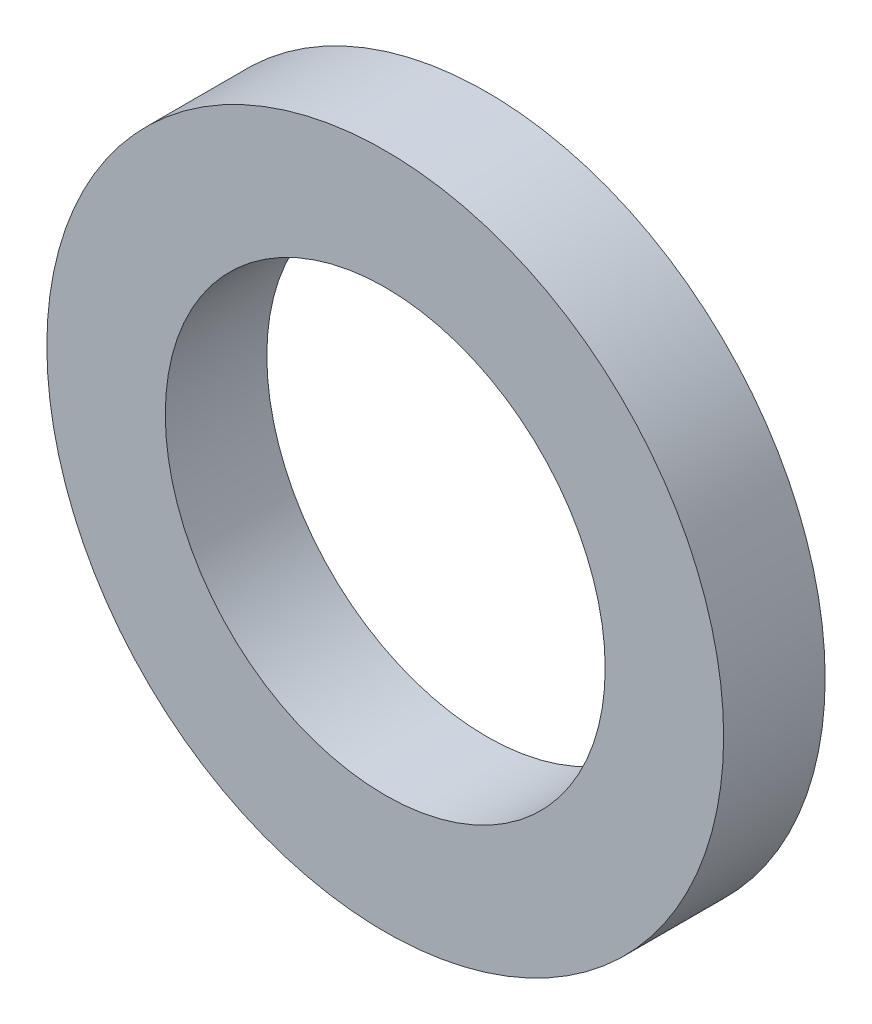
ISO-10303-21;
HEADER;
FILE_DESCRIPTION(('STEP AP214'),'2;1');
FILE_NAME('part.step','',(''),(''),'','','');
FILE_SCHEMA(('AUTOMOTIVE_DESIGN { 1 0 10303 214 1 1 1 1 }'));
ENDSEC;
DATA;
#1=APPLICATION_CONTEXT('core data for automotive mechanical design processes');
#2=APPLICATION_PROTOCOL_DEFINITION('international standard','automotive_design',2000,#1);
#3=PRODUCT_CONTEXT('',#1,'mechanical');
#4=PRODUCT('Part','Part','',(#3));
#5=PRODUCT_RELATED_PRODUCT_CATEGORY('part','',(#4));
#6=PRODUCT_DEFINITION_FORMATION('','',#4);
#7=PRODUCT_DEFINITION_CONTEXT('part definition',#1,'design');
#8=PRODUCT_DEFINITION('design','',#6,#7);
#9=PRODUCT_DEFINITION_SHAPE('','',#8);
#10=(LENGTH_UNIT() NAMED_UNIT(*) SI_UNIT(.MILLI.,.METRE.));
#11=(NAMED_UNIT(*) PLANE_ANGLE_UNIT() SI_UNIT($,.RADIAN.));
#12=(NAMED_UNIT(*) SI_UNIT($,.STERADIAN.) SOLID_ANGLE_UNIT());
#13=UNCERTAINTY_MEASURE_WITH_UNIT(LENGTH_MEASURE(1.E-05),#10,'distance_accuracy_value','');
#14=(GEOMETRIC_REPRESENTATION_CONTEXT(3) GLOBAL_UNCERTAINTY_ASSIGNED_CONTEXT((#13)) GLOBAL_UNIT_ASSIGNED_CONTEXT((#10,
#11,#12)) REPRESENTATION_CONTEXT('',''));
#15=CARTESIAN_POINT('',(0.,0.,0.));
#16=DIRECTION('',(0.,0.,1.));
#17=DIRECTION('',(1.,0.,0.));
#18=AXIS2_PLACEMENT_3D('',#15,#16,#17);
#19=CARTESIAN_POINT('',(0.,0.,3.));
#20=DIRECTION('',(0.,0.,1.));
#21=DIRECTION('',(1.,0.,0.));
#22=AXIS2_PLACEMENT_3D('',#19,#20,#21);
#23=PLANE('',#22);
#24=CARTESIAN_POINT('',(0.,0.,3.));
#25=DIRECTION('',(0.,0.,1.));
#26=DIRECTION('',(1.,0.,0.));
#27=AXIS2_PLACEMENT_3D('',#24,#25,#26);
#28=CIRCLE('',#27,10.);
#29=CARTESIAN_POINT('',(10.,0.,3.));
#30=VERTEX_POINT('',#29);
#31=EDGE_CURVE('E10',#30,#30,#28,.T.);
#32=ORIENTED_EDGE('',*,*,#31,.T.);
#33=EDGE_LOOP('',(#32));
#34=FACE_BOUND('',#33,.T.);
#35=CARTESIAN_POINT('',(0.,0.,3.));
#36=DIRECTION('',(0.,0.,1.));
#37=DIRECTION('',(1.,0.,0.));
#38=AXIS2_PLACEMENT_3D('',#35,#36,#37);
#39=CIRCLE('',#38,6.5);
#40=CARTESIAN_POINT('',(6.5,0.,3.));
#41=VERTEX_POINT('',#40);
#42=EDGE_CURVE('E49',#41,#41,#39,.T.);
#43=ORIENTED_EDGE('',*,*,#42,.F.);
#44=EDGE_LOOP('',(#43));
#45=FACE_BOUND('',#44,.T.);
#46=ADVANCED_FACE('F39',(#34,#45),#23,.T.);
#47=CARTESIAN_POINT('',(0.,0.,0.));
#48=DIRECTION('',(0.,0.,1.));
#49=DIRECTION('',(1.,0.,0.));
#50=AXIS2_PLACEMENT_3D('',#47,#48,#49);
#51=PLANE('',#50);
#52=CARTESIAN_POINT('',(0.,0.,0.));
#53=DIRECTION('',(0.,0.,1.));
#54=DIRECTION('',(1.,0.,0.));
#55=AXIS2_PLACEMENT_3D('',#52,#53,#54);
#56=CIRCLE('',#55,10.);
#57=CARTESIAN_POINT('',(10.,0.,0.));
#58=VERTEX_POINT('',#57);
#59=EDGE_CURVE('E43',#58,#58,#56,.T.);
#60=ORIENTED_EDGE('',*,*,#59,.F.);
#61=EDGE_LOOP('',(#60));
#62=FACE_BOUND('',#61,.T.);
#63=CARTESIAN_POINT('',(0.,0.,0.));
#64=DIRECTION('',(0.,0.,1.));
#65=DIRECTION('',(1.,0.,0.));
#66=AXIS2_PLACEMENT_3D('',#63,#64,#65);
#67=CIRCLE('',#66,6.5);
#68=CARTESIAN_POINT('',(6.5,0.,0.));
#69=VERTEX_POINT('',#68);
#70=EDGE_CURVE('E55',#69,#69,#67,.T.);
#71=ORIENTED_EDGE('',*,*,#70,.T.);
#72=EDGE_LOOP('',(#71));
#73=FACE_BOUND('',#72,.T.);
#74=ADVANCED_FACE('F64',(#62,#73),#51,.F.);
#75=CARTESIAN_POINT('',(0.,0.,3.));
#76=DIRECTION('',(0.,0.,-1.));
#77=DIRECTION('',(-1.,0.,0.));
#78=AXIS2_PLACEMENT_3D('',#75,#76,#77);
#79=CYLINDRICAL_SURFACE('',#78,10.);
#80=ORIENTED_EDGE('',*,*,#31,.F.);
#81=EDGE_LOOP('',(#80));
#82=FACE_BOUND('',#81,.T.);
#83=ORIENTED_EDGE('',*,*,#59,.T.);
#84=EDGE_LOOP('',(#83));
#85=FACE_BOUND('',#84,.T.);
#86=ADVANCED_FACE('F41',(#82,#85),#79,.T.);
#87=CARTESIAN_POINT('',(0.,0.,3.));
#88=DIRECTION('',(0.,0.,-1.));
#89=DIRECTION('',(-1.,0.,0.));
#90=AXIS2_PLACEMENT_3D('',#87,#88,#89);
#91=CYLINDRICAL_SURFACE('',#90,6.5);
#92=ORIENTED_EDGE('',*,*,#42,.T.);
#93=EDGE_LOOP('',(#92));
#94=FACE_BOUND('',#93,.T.);
#95=ORIENTED_EDGE('',*,*,#70,.F.);
#96=EDGE_LOOP('',(#95));
#97=FACE_BOUND('',#96,.T.);
#98=ADVANCED_FACE('F59',(#94,#97),#91,.F.);
#99=CLOSED_SHELL('',(#46,#74,#86,#98));
#100=MANIFOLD_SOLID_BREP('B2',#99);
#101=ADVANCED_BREP_SHAPE_REPRESENTATION('',(#18,#100),#14);
#102=SHAPE_DEFINITION_REPRESENTATION(#9,#101);
ENDSEC;
END-ISO-10303-21;
